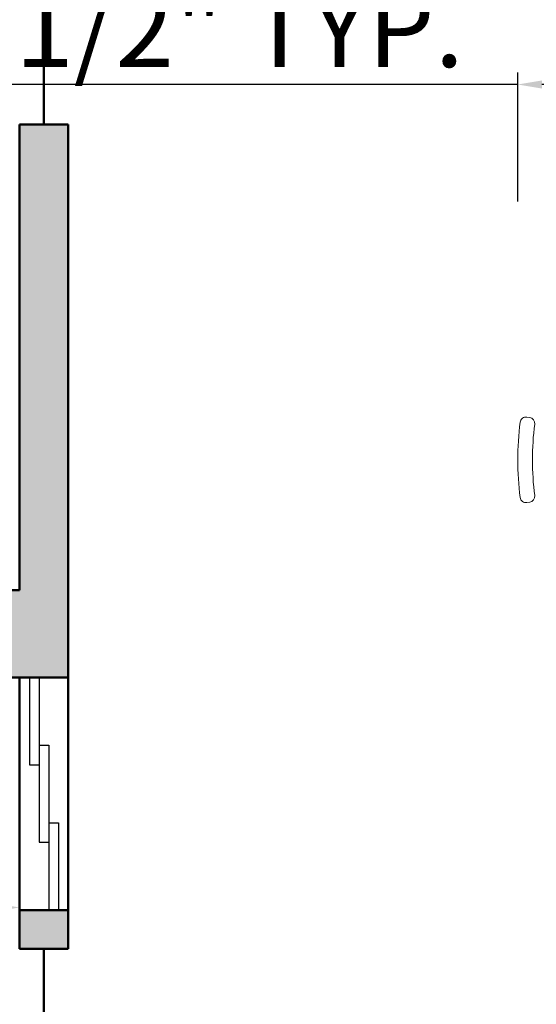
# Model space of a CAD drawing. Units: inches. Extents: x 1913 to 5309, y 1003 to 1733.
# Tile 16 of 23: x 4152 to 4205, y 1387 to 1489. Entities that reach past the tile are written whole.
import ezdxf

# ---------------------------------------------------------------- set-up
doc = ezdxf.new("R2010")
doc.units = ezdxf.units.IN
for name, color, linetype, lineweight in [('A-ANNO-DIMS', 2, 'Continuous', 18), ('A-FLOR-PATT', 252, 'Continuous', 13), ('A-FURN', 8, 'Continuous', 18), ('A-GLAZ', 5, 'Continuous', 25), ('A-WALL', 7, 'Continuous', 50)]:
    doc.layers.add(name, color=color, linetype=linetype, lineweight=lineweight)
doc.styles.get("Standard").update_dxf_attribs({"font": 'arial.ttf'})
doc.dimstyles.new('ISO-25', dxfattribs={"dimtxt": 8, "dimasz": 2.5, "dimexe": 1.25, "dimexo": 0.625, "dimtad": 1, "dimdec": 1, "dimlunit": 3, "dimtxsty": 'Standard', "dimcen": 2.5, "dimclrd": 256, "dimclrt": 1, "dimadec": 0, "dimazin": 0, "dimtfac": 1, "dimtdec": 1, "dimtmove": 0, "dimatfit": 3, "dimfxl": 1, "dimarcsym": 0})

# ---------------------------------------------------------------- blocks, each defined once
blk = doc.blocks.new('A$C421907B3')
at = {"ltscale": 0.1}
blk.add_lwpolyline([(0.9489, 2.7478, 0.030867), (0.827, 2.7403, -0.408428), (0.8047, 2.7573), (0.8033, 2.7672, -0.419966), (0.8206, 2.7899, -0.030916), (0.9489, 2.7978, -0.030916), (1.0772, 2.7899, -0.419966), (1.0945, 2.7672), (1.0931, 2.7573, -0.408428), (1.0708, 2.7403, 0.030867)], format="xyb", close=True, dxfattribs=at)
blk = doc.blocks.new('*D36')
at = {"layer": 'A-ANNO-DIMS', "color": 0, "lineweight": -2, "transparency": 16777216}
for p, q in [((3999.21, 1406.34), (3999.21, 1395.99)), ((4152.21, 1406.34), (4152.21, 1395.99)), ((4149.71, 1397.24), (4001.71, 1397.24))]:
    blk.add_line(p, q, dxfattribs=at)
at = {"layer": 'A-ANNO-DIMS', "color": 0, "transparency": 16777216}
for points in [[(4001.71, 1397.65), (4001.71, 1396.82), (3999.21, 1397.24)], [(4149.71, 1397.65), (4149.71, 1396.82), (4152.21, 1397.24)]]:
    blk.add_solid(points, dxfattribs=at)
at = {"layer": 'Defpoints', "color": 0, "transparency": 16777216}
for p in [(3999.21, 1406.96), (4152.21, 1406.96), (3999.21, 1397.24)]:
    blk.add_point(p, dxfattribs=at)
at = {"layer": 'A-ANNO-DIMS', "color": 0, "transparency": 16777216, "insert": (4075.71, 1401.95), "char_height": 8, "attachment_point": 5}
blk.add_mtext('12\'-9"', dxfattribs=at)
blk = doc.blocks.new('WIN-24')
for p, q in [((0, 15), (0, 24)), ((1, 7), (1, 24)), ((2, 17), (1, 17)), ((2, 0), (2, 17)), ((1, 15), (0, 15)), ((3, 9), (2, 9)), ((3, 0), (3, 9)), ((2, 7), (1, 7))]:
    blk.add_line(p, q)
blk = doc.blocks.new('*D83')
at = {"layer": 'A-ANNO-DIMS', "color": 0, "lineweight": -2, "transparency": 16777216}
for p, q in [((4203.55, 1470.03), (4203.55, 1483.35)), ((4288.22, 1470.03), (4288.22, 1483.35))]:
    blk.add_line(p, q, dxfattribs=at)
at = {"layer": 'A-ANNO-DIMS', "lineweight": -2, "transparency": 16777216}
for p, q in [((4203.55, 1482.1), (4065.74, 1482.1)), ((4285.72, 1482.1), (4206.05, 1482.1))]:
    blk.add_line(p, q, dxfattribs=at)
at = {"layer": 'A-ANNO-DIMS', "transparency": 16777216}
for points in [[(4206.05, 1482.52), (4206.05, 1481.68), (4203.55, 1482.1)], [(4285.72, 1482.52), (4285.72, 1481.68), (4288.22, 1482.1)]]:
    blk.add_solid(points, dxfattribs=at)
at = {"layer": 'Defpoints', "color": 0, "transparency": 16777216}
for p in [(4203.55, 1482.1), (4203.55, 1469.4), (4288.22, 1469.4)]:
    blk.add_point(p, dxfattribs=at)
at = {"layer": 'A-ANNO-DIMS', "color": 1, "transparency": 16777216, "insert": (4133.4, 1486.86), "char_height": 8, "attachment_point": 5}
blk.add_mtext('DINING SET 7\'-0 1/2" TYP.', dxfattribs=at)

msp = doc.modelspace()

# ---------------------------------------------------------------- hatches: boundary and pattern name
at = {"layer": 'A-FLOR-PATT'}
h = msp.add_hatch(color=256, dxfattribs=at)
h.dxf.hatch_style = 1
h.paths.add_polyline_path([(4179.21, 1155.93), (4164.35, 1155.93, -0.035946), (4163.9, 1155.96), (4161.21, 1155.96), (4161.21, 1173.96), (4152.21, 1173.96), (4152.21, 1146.96), (4179.21, 1146.96)])
h.paths.add_polyline_path([(4273.21, 1155.96), (4266.93, 1155.96), (4233.21, 1155.96), (4233.21, 1146.96), (4273.21, 1146.96)])
h.paths.add_polyline_path([(4285.21, 1328.96), (4152.21, 1328.96), (4152.21, 1305.96), (4161.21, 1305.96), (4161.21, 1323.96), (4285.21, 1323.96)])
h.paths.add_polyline_path([(4161.21, 1257.96), (4152.21, 1257.96), (4152.21, 1233.96), (4161.21, 1233.96), (4161.21, 1237.71)])
h.paths.add_polyline_path([(4515.21, 1405.96), (4503.21, 1405.96), (4503.21, 1400.96), (4506.21, 1400.96), (4506.21, 1328.96), (4452.21, 1328.96), (4452.21, 1323.96), (4506.21, 1323.96), (4506.21, 1179.96), (4455.21, 1179.96), (4455.21, 1170.96), (4515.21, 1170.96)])
h.paths.add_polyline_path([(4157.21, 1686.96), (3999.21, 1686.96), (3999.21, 1625.96), (4008.21, 1625.96), (4008.21, 1677.96), (4152.21, 1677.96), (4152.21, 1554.96), (4157.21, 1554.96), (4157.21, 1599.96), (4225.21, 1599.96), (4225.21, 1608.96), (4157.21, 1608.96)])
h.paths.add_polyline_path([(4008.21, 1513.96), (4157.21, 1513.96), (4157.21, 1518.96), (4008.21, 1518.96), (4008.21, 1571.96), (3999.21, 1571.96), (3999.21, 1420.96), (4050.21, 1420.96), (4050.21, 1429.96), (4008.21, 1429.96)])
h.paths.add_polyline_path([(4157.21, 1477.96), (4152.21, 1477.96), (4152.21, 1429.96), (4110.21, 1429.96), (4110.21, 1420.96), (4157.21, 1420.96)], flags=17)
h.paths.add_polyline_path([(4350.21, 1608.96), (4345.21, 1608.96), (4321.21, 1608.96), (4321.21, 1599.96), (4350.21, 1599.96)])
h.paths.add_polyline_path([(4515.21, 1686.96), (4345.21, 1686.96), (4345.21, 1644.96), (4350.21, 1644.96), (4350.21, 1677.96), (4506.21, 1677.96), (4506.21, 1557.96), (4423.21, 1557.96), (4423.21, 1552.96), (4506.21, 1552.96), (4506.21, 1492.96), (4428.21, 1492.96), (4428.21, 1522.96), (4423.21, 1522.96), (4423.21, 1492.96), (4345.21, 1492.96), (4345.21, 1487.96), (4474.21, 1487.96), (4474.21, 1464.96), (4479.21, 1464.96), (4479.21, 1487.96), (4515.21, 1487.96)])
h.paths.add_polyline_path([(4479.21, 1428.96), (4474.21, 1428.96), (4474.21, 1405.96), (4345.21, 1405.96), (4345.21, 1358.96), (4350.21, 1358.96), (4350.21, 1400.96), (4417.21, 1400.96), (4417.21, 1394.96), (4422.21, 1394.96), (4422.21, 1400.96), (4479.21, 1400.96)])
h.paths.add_polyline_path([(4350.21, 1323.96), (4422.21, 1323.96), (4422.21, 1370.96), (4417.21, 1370.96), (4417.21, 1328.96), (4345.21, 1328.96), (4345.21, 1158.97, -0.414214), (4342.21, 1155.96), (4327.21, 1155.96), (4327.21, 1146.96), (4350.21, 1146.96), (4350.21, 1170.96), (4401.21, 1170.96), (4401.21, 1179.96), (4350.21, 1179.96)])
h.paths.add_polyline_path([(4157.21, 1356.96), (4152.21, 1356.96), (4152.21, 1352.96), (4157.21, 1352.96)])
h.paths.add_polyline_path([(4157.21, 1396.96), (4152.21, 1396.96), (4152.21, 1392.96), (4157.21, 1392.96)])

# ---------------------------------------------------------------- linework, layer by layer
at = {"layer": 'A-WALL'}
for p, q in [((4154.71, 1513.96), (4154.71, 1477.96)), ((4152.21, 1477.96), (4152.21, 1429.96)), ((4152.21, 1477.96), (4157.21, 1477.96)), ((4157.21, 1477.96), (4157.21, 1392.96)), ((4008.21, 1429.96), (4152.21, 1429.96)), ((3999.21, 1420.96), (4157.21, 1420.96)), ((4152.21, 1420.96), (4152.21, 1392.96)), ((4152.21, 1396.96), (4157.21, 1396.96)), ((4152.21, 1392.96), (4157.21, 1392.96)), ((4154.71, 1392.96), (4154.71, 1356.96))]:
    msp.add_line(p, q, dxfattribs=at)

# ---------------------------------------------------------------- block references
at = {"layer": 'A-FURN', "xscale": 30.26057373645948, "yscale": 30.26057373645948, "zscale": 30.26057373645948, "rotation": 89.99999999999996}
msp.add_blockref('A$C421907B3', (4288.22, 1414.68), dxfattribs=at)
at = {"layer": 'A-GLAZ', "rotation": 180}
msp.add_blockref('WIN-24', (4156.21, 1420.96), dxfattribs=at)

# ---------------------------------------------------------------- dimensions: what is measured, and where the dimension line sits
at = {"layer": 'A-ANNO-DIMS'}
dim = msp.add_linear_dim(base=(4203.55, 1482.1), p1=(4288.22, 1469.4), p2=(4203.55, 1469.4), angle=180, text='DINING SET <> TYP.', dimstyle='ISO-25', override={"dimdec": 1, "dimrnd": 0, "dimzin": 1, "dimlunit": 4, "dimfrac": 2}, dxfattribs=at)
dim.commit()
dim.dimension.update_dxf_attribs({"geometry": '*D83', "text_midpoint": (4133.4, 1486.86)})
dim = msp.add_linear_dim(base=(3999.21, 1397.24), p1=(4152.21, 1406.96), p2=(3999.21, 1406.96), dimstyle='ISO-25', override={"dimclrd": 0, "dimclre": 0, "dimclrt": 0}, dxfattribs=at)
dim.commit()
dim.dimension.update_dxf_attribs({"geometry": '*D36', "text_midpoint": (4075.71, 1401.95)})

doc.saveas('drawing.dxf')
